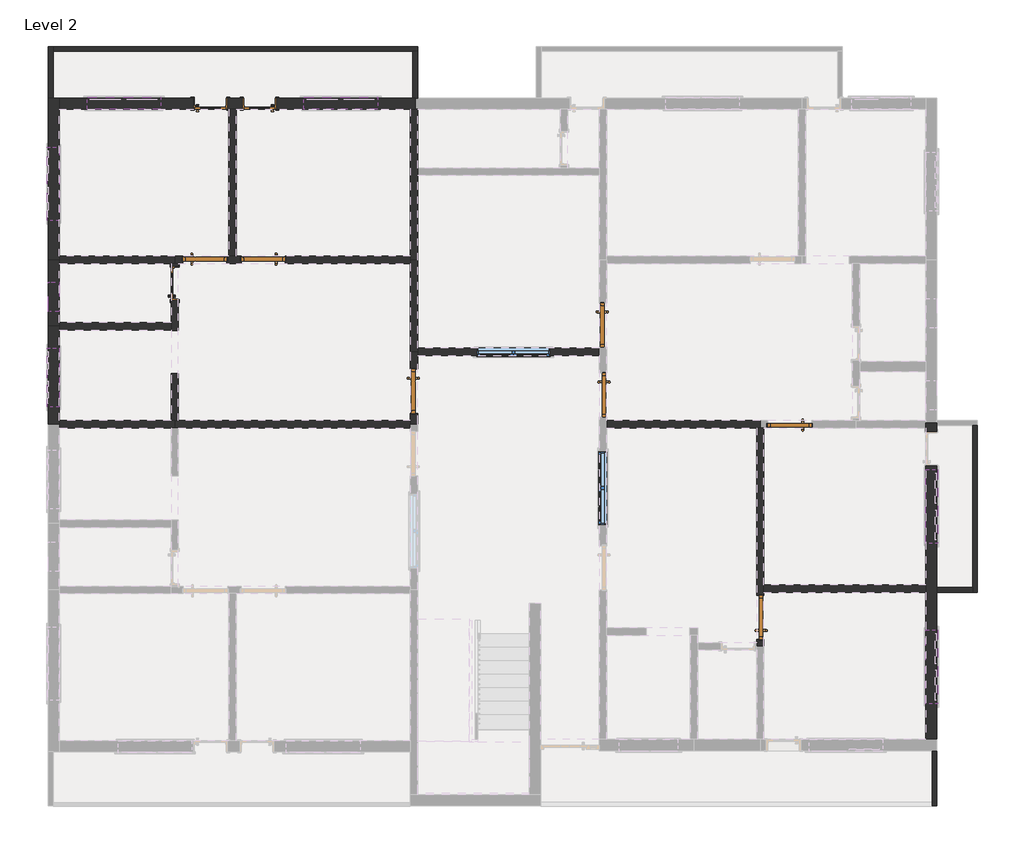
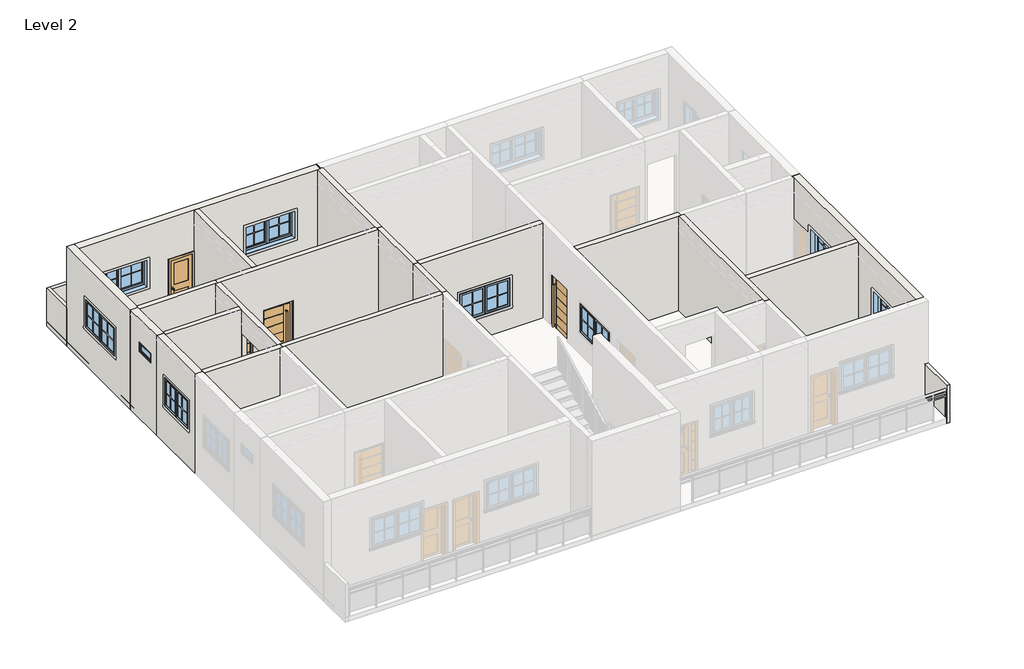
# One storey, part 2 of 5: 25 walls, 10 doors, 9 windows.
"""IFC4 building model written with IfcOpenShell, lengths in millimetres."""

from ifc_helpers import new_model, si_unit, frame, origin, place, context, project, spatial, polyline, outline, extrude, faceted_brep, transform, mapped, element, save
from components import door_3_ad1505b7, door_3_44036f4b, door_57d9c04c, door_5f4ff63b, door_e2914254, fixed_2_d9cafb20, m_window_awning_double_horizontal_4_0c6a2509, m_window_awning_double_horizontal_5_7c720334, m_window_awning_double_horizontal_5_337400f2

model = new_model("IFC4")

# Units and contexts
model_context = context("Model", 3, world=origin())
ifc_project = project(units=[si_unit("LENGTHUNIT", "METRE", prefix="MILLI")], contexts=[model_context])

# Site, building, storey
site = spatial("IfcSite", under=ifc_project)
building = spatial("IfcBuilding", under=site)
storey = spatial("IfcBuildingStorey", under=building, Name="Level 2", Elevation=3200.4)

# Doors
placement = place(None, origin())
door_3_shape = door_3_ad1505b7(model_context)
element("IfcDoor", 1, ObjectType="3'", at=placement, inside=storey, context=model_context, shape_type="MappedRepresentation", body=[
    mapped(door_3_shape, transform((-21766.1847893, 19978.1922903, 3200.4), x_axis=(1.0, 0.0, 0.0), y_axis=(0.0, 1.0, 0.0), z_axis=(0.0, 0.0, 1.0))),
])
element("IfcDoor", 2, ObjectType="3'", at=placement, inside=storey, context=model_context, shape_type="MappedRepresentation", body=[
    mapped(door_3_shape, transform((-13523.8847893, 17184.1922903, 3200.4), x_axis=(0.0, -1.0, 0.0), y_axis=(1.0, 0.0, 0.0), z_axis=(0.0, 0.0, 1.0))),
])
element("IfcDoor", 3, ObjectType="3'", at=placement, inside=storey, context=model_context, shape_type="MappedRepresentation", body=[
    mapped(door_3_shape, transform((-9663.0847893, 16574.5922903, 3200.4), x_axis=(-1.0, 0.0, 0.0), y_axis=(0.0, -1.0, 0.0), z_axis=(0.0, 0.0, 1.0))),
])
door_3_2_shape = door_3_44036f4b(model_context)
element("IfcDoor", 4, ObjectType="3'", at=placement, inside=storey, context=model_context, shape_type="MappedRepresentation", body=[
    mapped(door_3_2_shape, transform((-20559.6847893, 19978.1922903, 3200.4), x_axis=(-1.0, 0.0, 0.0), y_axis=(0.0, -1.0, 0.0), z_axis=(0.0, 0.0, 1.0))),
])
element("IfcDoor", 5, ObjectType="3'", at=placement, inside=storey, context=model_context, shape_type="MappedRepresentation", body=[
    mapped(door_3_2_shape, transform((-17435.4847893, 17260.3922903, 3200.4), x_axis=(0.0, -1.0, 0.0), y_axis=(1.0, 0.0, 0.0), z_axis=(0.0, 0.0, 1.0))),
])
element("IfcDoor", 6, ObjectType="3'", at=placement, inside=storey, context=model_context, shape_type="MappedRepresentation", body=[
    mapped(door_3_2_shape, transform((-13523.8847893, 18631.9922903, 3200.4), x_axis=(0.0, -1.0, 0.0), y_axis=(1.0, 0.0, 0.0), z_axis=(0.0, 0.0, 1.0))),
])
element("IfcDoor", 7, ObjectType="3'", at=placement, inside=storey, context=model_context, shape_type="MappedRepresentation", body=[
    mapped(door_3_2_shape, transform((-10272.6847893, 12574.0922903, 3200.4), x_axis=(0.0, 1.0, 0.0), y_axis=(-1.0, 0.0, 0.0), z_axis=(0.0, 0.0, 1.0))),
])
door_shape = door_57d9c04c(model_context)
element("IfcDoor", 8, ObjectType="M_Door-Interior-Single-2_Panel-Wood : 2'2\"", at=placement, inside=storey, context=model_context, shape_type="MappedRepresentation", body=[
    mapped(door_shape, transform((-22391.6597893, 19495.5922903, 3200.4), x_axis=(0.0, 1.0, 0.0), y_axis=(-1.0, 0.0, 0.0), z_axis=(0.0, 0.0, 1.0))),
])
door_2_shape = door_5f4ff63b(model_context)
element("IfcDoor", 9, ObjectType="M_Door-Interior-Single-2_Panel-Wood : 2'2\"", at=placement, inside=storey, context=model_context, shape_type="MappedRepresentation", body=[
    mapped(door_2_shape, transform((-20635.8847893, 23213.5172903, 3200.4), x_axis=(-1.0, 0.0, 0.0), y_axis=(0.0, -1.0, 0.0), z_axis=(0.0, 0.0, 1.0))),
])
door_4_shape = door_e2914254(model_context)
element("IfcDoor", 10, ObjectType="M_Door-Interior-Single-2_Panel-Wood : 2'2\"", at=placement, inside=storey, context=model_context, shape_type="MappedRepresentation", body=[
    mapped(door_4_shape, transform((-21651.8847893, 23213.5172903, 3200.4), x_axis=(1.0, 0.0, 0.0), y_axis=(0.0, 1.0, 0.0), z_axis=(0.0, 0.0, 1.0))),
])

# Walls
element("IfcWall", 11, ObjectType="Generic - 4\"", at=placement, inside=storey, context=model_context, shape_type="Brep", body=[
    faceted_brep([(-24903.0847893, 23330.9922903, 3200.4), (-24903.0847893, 24296.1922903, 3200.4), (-24903.0847893, 24397.7922903, 3200.4), (-24903.0847893, 24397.7922903, 4419.6), (-24903.0847893, 24296.1922903, 4419.6), (-24903.0847893, 23330.9922903, 4419.6), (-25004.6847893, 23330.9922903, 3200.4), (-25004.6847893, 23330.9922903, 4419.6), (-25004.6847893, 24397.7922903, 4419.6), (-25004.6847893, 24397.7922903, 3200.4)], [[[0, 1, 2, 3, 4, 5]], [[6, 7, 8, 9]], [[2, 1, 0, 6, 9]], [[5, 4, 3, 8, 7]], [[0, 5, 7, 6]], [[3, 2, 9, 8]]]),
])
element("IfcWall", 12, ObjectType="Generic - 4\"", at=placement, inside=storey, context=model_context, shape_type="Brep", body=[
    faceted_brep([(-24903.0847893, 24296.1922903, 3200.4), (-17460.8847893, 24296.1922903, 3200.4), (-17359.2847893, 24296.1922903, 3200.4), (-17359.2847893, 24296.1922903, 4419.6), (-17460.8847893, 24296.1922903, 4419.6), (-24903.0847893, 24296.1922903, 4419.6), (-24903.0847893, 24397.7922903, 3200.4), (-24903.0847893, 24397.7922903, 4419.6), (-17359.2847893, 24397.7922903, 4419.6), (-17359.2847893, 24397.7922903, 3200.4)], [[[0, 1, 2, 3, 4, 5]], [[6, 7, 8, 9]], [[2, 1, 0, 6, 9]], [[5, 4, 3, 8, 7]], [[0, 5, 7, 6]], [[3, 2, 9, 8]]]),
])
element("IfcWall", 13, ObjectType="Generic - 4\"", at=placement, inside=storey, context=model_context, shape_type="Brep", body=[
    faceted_brep([(-17460.8847893, 24296.1922903, 3200.4), (-17460.8847893, 23330.9922903, 3200.4), (-17460.8847893, 23330.9922903, 4419.6), (-17460.8847893, 24296.1922903, 4419.6), (-17359.2847893, 24296.1922903, 3200.4), (-17359.2847893, 24296.1922903, 4419.6), (-17359.2847893, 23330.9922903, 4419.6), (-17359.2847893, 23330.9922903, 3200.4), (-17410.0847893, 23330.9922903, 3200.4), (-17435.4847893, 23330.9922903, 3200.4)], [[[0, 1, 2, 3]], [[4, 5, 6, 7]], [[1, 0, 4, 7, 8, 9]], [[3, 2, 6, 5]], [[0, 3, 5, 4]], [[2, 1, 9, 8, 7, 6]]]),
])
element("IfcWall", 14, ObjectType="Generic - 4\"", at=placement, inside=storey, context=model_context, shape_type="Brep", body=[
    faceted_brep([(-5878.4847893, 16549.1922903, 3200.4), (-5878.4847893, 13196.3922903, 3200.4), (-5878.4847893, 13094.7922903, 3200.4), (-5878.4847893, 13094.7922903, 4419.6), (-5878.4847893, 13196.3922903, 4419.6), (-5878.4847893, 16549.1922903, 4419.6), (-5776.8847893, 16549.1922903, 3200.4), (-5776.8847893, 16549.1922903, 4419.6), (-5776.8847893, 13094.7922903, 4419.6), (-5776.8847893, 13094.7922903, 3200.4)], [[[0, 1, 2, 3, 4, 5]], [[6, 7, 8, 9]], [[2, 1, 0, 6, 9]], [[5, 4, 3, 8, 7]], [[0, 5, 7, 6]], [[3, 2, 9, 8]]]),
])
element("IfcWall", 15, ObjectType="Generic - 4\"", at=placement, inside=storey, context=model_context, shape_type="SweptSolid", body=[
    extrude(outline(polyline([(-6615.0847893, 13196.3922903), (-5878.4847893, 13196.3922903), (-5878.4847893, 13094.7922903), (-6615.0847893, 13094.7922903), (-6615.0847893, 13196.3922903)])), frame((0.0, 0.0, 3200.4), z_axis=(0.0, 0.0, 1.0), x_axis=(1.0, 0.0, 0.0)), (0.0, 0.0, 1.0), 1219.2),
])
element("IfcWall", 16, ObjectType="Generic - 4\"", at=placement, inside=storey, context=model_context, shape_type="SweptSolid", body=[
    extrude(outline(polyline([(-6716.6847893, 8675.1922903), (-6716.6847893, 9818.1922903), (-6615.0847893, 9818.1922903), (-6615.0847893, 8675.1922903), (-6716.6847893, 8675.1922903)])), frame((0.0, 0.0, 3200.4), z_axis=(0.0, 0.0, 1.0), x_axis=(1.0, 0.0, 0.0)), (0.0, 0.0, 1.0), 1219.2),
])
element("IfcWall", 17, ObjectType="Generic - 6\"", at=placement, inside=storey, context=model_context, shape_type="Brep", body=[
    faceted_brep([(-17511.6847893, 23102.3922903, 6400.8), (-17511.6847893, 23102.3922903, 3200.4), (-17511.6847893, 20054.3922903, 3200.4), (-17511.6847893, 19978.1922903, 3200.4), (-17511.6847893, 19978.1922903, 6400.8), (-17511.6847893, 20054.3922903, 6400.8), (-17359.2847893, 23102.3922903, 3200.4), (-17359.2847893, 23102.3922903, 6400.8), (-17359.2847893, 21883.1922903, 6400.8), (-17359.2847893, 21730.7922903, 6400.8), (-17359.2847893, 19978.1922903, 6400.8), (-17359.2847893, 19978.1922903, 3200.4), (-17359.2847893, 21730.7922903, 3200.4), (-17359.2847893, 21883.1922903, 3200.4), (-17435.4847893, 23102.3922903, 3200.4), (-17410.0847893, 23102.3922903, 3200.4), (-17410.0847893, 23102.3922903, 6400.8), (-17435.4847893, 23102.3922903, 6400.8)], [[[0, 1, 2, 3, 4, 5]], [[6, 7, 8, 9, 10, 11, 12, 13]], [[3, 2, 1, 14, 15, 6, 13, 12, 11]], [[4, 3, 11, 10]], [[0, 5, 4, 10, 9, 8, 7, 16, 17]], [[0, 17, 16, 7, 6, 15, 14, 1]]]),
])
element("IfcWall", 18, ObjectType="Generic - 6\"", at=placement, inside=storey, context=model_context, shape_type="Brep", body=[
    faceted_brep([(-24776.0847893, 19901.9922903, 3200.4), (-22464.6847893, 19901.9922903, 3200.4), (-22388.4847893, 19901.9922903, 3200.4), (-22388.4847893, 19901.9922903, 6400.8), (-22464.6847893, 19901.9922903, 6400.8), (-24776.0847893, 19901.9922903, 6400.8), (-24776.0847893, 20054.3922903, 3200.4), (-24776.0847893, 20054.3922903, 6400.8), (-22388.4847893, 20054.3922903, 6400.8), (-22388.4847893, 20054.3922903, 3200.4), (-24776.0847893, 19978.1922903, 3200.4), (-24776.0847893, 19978.1922903, 6400.8)], [[[0, 1, 2, 3, 4, 5]], [[6, 7, 8, 9]], [[2, 1, 0, 10, 6, 9]], [[3, 2, 9, 8]], [[5, 4, 3, 8, 7, 11]], [[0, 5, 11, 7, 6, 10]]]),
])
element("IfcWall", 19, ObjectType="Generic - 6\"", at=placement, inside=storey, context=model_context, shape_type="SweptSolid", body=[
    extrude(outline(polyline([(-21270.8847893, 20054.3922903), (-21270.8847893, 23102.3922903), (-21118.4847893, 23102.3922903), (-21118.4847893, 20054.3922903), (-21270.8847893, 20054.3922903)])), frame((0.0, 0.0, 3200.4), z_axis=(0.0, 0.0, 1.0), x_axis=(1.0, 0.0, 0.0)), (0.0, 0.0, 1.0), 3200.4),
])
element("IfcWall", 20, ObjectType="Generic - 6\"", at=placement, inside=storey, context=model_context, shape_type="Brep", body=[
    faceted_brep([(-24776.0847893, 16498.3922903, 3200.4), (-22464.6847893, 16498.3922903, 3200.4), (-22388.4847893, 16498.3922903, 3200.4), (-22388.4847893, 16498.3922903, 6400.8), (-22464.6847893, 16498.3922903, 6400.8), (-24776.0847893, 16498.3922903, 6400.8), (-24776.0847893, 16650.7922903, 3200.4), (-24776.0847893, 16650.7922903, 6400.8), (-22464.6847893, 16650.7922903, 6400.8), (-22388.4847893, 16650.7922903, 6400.8), (-22388.4847893, 16650.7922903, 3200.4), (-22464.6847893, 16650.7922903, 3200.4), (-24776.0847893, 16574.5922903, 3200.4), (-24776.0847893, 16574.5922903, 6400.8)], [[[0, 1, 2, 3, 4, 5]], [[6, 7, 8, 9, 10, 11]], [[2, 1, 0, 12, 6, 11, 10]], [[3, 2, 10, 9]], [[5, 4, 3, 9, 8, 7, 13]], [[0, 5, 13, 7, 6, 12]]]),
])
element("IfcWall", 21, ObjectType="Generic - 6\"", at=placement, inside=storey, context=model_context, shape_type="Brep", body=[
    faceted_brep([(-24776.0847893, 18530.3922903, 3200.4), (-22464.6847893, 18530.3922903, 3200.4), (-22464.6847893, 18530.3922903, 6400.8), (-24776.0847893, 18530.3922903, 6400.8), (-24776.0847893, 18682.7922903, 3200.4), (-24776.0847893, 18682.7922903, 6400.8), (-22464.6847893, 18682.7922903, 6400.8), (-22464.6847893, 18682.7922903, 3200.4), (-24776.0847893, 18606.5922903, 3200.4), (-24776.0847893, 18606.5922903, 6400.8)], [[[0, 1, 2, 3]], [[4, 5, 6, 7]], [[1, 0, 8, 4, 7]], [[3, 2, 6, 5, 9]], [[0, 3, 9, 5, 4, 8]], [[2, 1, 7, 6]]]),
])
element("IfcWall", 22, ObjectType="Generic - 6\"", at=placement, inside=storey, context=model_context, shape_type="Brep", body=[
    faceted_brep([(-22312.2847893, 19901.9922903, 6400.8), (-22312.2847893, 16650.7922903, 6400.8), (-22312.2847893, 16650.7922903, 3200.4), (-22312.2847893, 17622.2018411, 3200.4), (-22312.2847893, 17622.2018411, 5638.8), (-22312.2847893, 18518.7795946, 5638.8), (-22312.2847893, 18518.7795946, 3200.4), (-22312.2847893, 19140.3922903, 3200.4), (-22312.2847893, 19140.3922903, 5054.2), (-22312.2847893, 19850.7922903, 5054.2), (-22312.2847893, 19850.7922903, 3200.4), (-22312.2847893, 19901.9922903, 3200.4), (-22464.6847893, 16650.7922903, 6400.8), (-22464.6847893, 18530.3922903, 6400.8), (-22464.6847893, 18682.7922903, 6400.8), (-22464.6847893, 19901.9922903, 6400.8), (-22464.6847893, 19901.9922903, 3200.4), (-22464.6847893, 19850.7922903, 3200.4), (-22464.6847893, 19850.7922903, 5054.2), (-22464.6847893, 19140.3922903, 5054.2), (-22464.6847893, 19140.3922903, 3200.4), (-22464.6847893, 18682.7922903, 3200.4), (-22464.6847893, 18530.3922903, 3200.4), (-22464.6847893, 18518.7795946, 3200.4), (-22464.6847893, 18518.7795946, 5638.8), (-22464.6847893, 17622.2018411, 5638.8), (-22464.6847893, 17622.2018411, 3200.4), (-22464.6847893, 16650.7922903, 3200.4), (-22388.4847893, 16650.7922903, 3200.4), (-22388.4847893, 19901.9922903, 3200.4), (-22388.4847893, 19901.9922903, 6400.8), (-22388.4847893, 16650.7922903, 6400.8)], [[[0, 1, 2, 3, 4, 5, 6, 7, 8, 9, 10, 11]], [[12, 13, 14, 15, 16, 17, 18, 19, 20, 21, 22, 23, 24, 25, 26, 27]], [[2, 28, 27, 26, 3]], [[6, 23, 22, 21, 20, 7]], [[16, 29, 11, 10, 17]], [[1, 0, 30, 15, 14, 13, 12, 31]], [[0, 11, 29, 16, 15, 30]], [[2, 1, 31, 12, 27, 28]], [[9, 18, 17, 10]], [[18, 9, 8, 19]], [[19, 8, 7, 20]], [[4, 25, 24, 5]], [[25, 4, 3, 26]], [[5, 24, 23, 6]]]),
])
element("IfcWall", 23, ObjectType="Generic - 6\"", at=placement, inside=storey, context=model_context, shape_type="Brep", body=[
    faceted_brep([(-17359.2847893, 17996.9922903, 3200.4), (-13600.0847893, 17996.9922903, 3200.4), (-13600.0847893, 17996.9922903, 6400.8), (-17359.2847893, 17996.9922903, 6400.8), (-16140.0847893, 17996.9922903, 5014.8), (-14616.0847893, 17996.9922903, 5014.8), (-14616.0847893, 17996.9922903, 4100.4), (-16140.0847893, 17996.9922903, 4100.4), (-17359.2847893, 18149.3922903, 3200.4), (-17359.2847893, 18149.3922903, 6400.8), (-13600.0847893, 18149.3922903, 6400.8), (-13600.0847893, 18149.3922903, 3200.4), (-16140.0847893, 18149.3922903, 5014.8), (-16140.0847893, 18149.3922903, 4100.4), (-14616.0847893, 18149.3922903, 4100.4), (-14616.0847893, 18149.3922903, 5014.8), (-17359.2847893, 18073.1922903, 3200.4), (-17359.2847893, 18073.1922903, 6400.8)], [[[0, 1, 2, 3], [4, 5, 6, 7]], [[8, 9, 10, 11], [12, 13, 14, 15]], [[1, 0, 16, 8, 11]], [[3, 2, 10, 9, 17]], [[0, 3, 17, 9, 8, 16]], [[2, 1, 11, 10]], [[13, 12, 4, 7]], [[14, 13, 7, 6]], [[15, 14, 6, 5]], [[12, 15, 5, 4]]]),
])
element("IfcWall", 24, ObjectType="Generic - 6\"", at=placement, inside=storey, context=model_context, shape_type="Brep", body=[
    faceted_brep([(-13447.6847893, 16498.3922903, 3200.4), (-10348.8847893, 16498.3922903, 3200.4), (-10272.6847893, 16498.3922903, 3200.4), (-10272.6847893, 16498.3922903, 6400.8), (-10348.8847893, 16498.3922903, 6400.8), (-13447.6847893, 16498.3922903, 6400.8), (-13447.6847893, 16650.7922903, 3200.4), (-13447.6847893, 16650.7922903, 6400.8), (-10272.6847893, 16650.7922903, 6400.8), (-10272.6847893, 16650.7922903, 3200.4)], [[[0, 1, 2, 3, 4, 5]], [[6, 7, 8, 9]], [[2, 1, 0, 6, 9]], [[3, 2, 9, 8]], [[5, 4, 3, 8, 7]], [[0, 5, 7, 6]]]),
])
element("IfcWall", 25, ObjectType="Generic - 6\"", at=placement, inside=storey, context=model_context, shape_type="Brep", body=[
    faceted_brep([(-10348.8847893, 11977.1922903, 3200.4), (-10348.8847893, 11977.1922903, 6400.8), (-10348.8847893, 12053.3922903, 6400.8), (-10348.8847893, 16498.3922903, 6400.8), (-10348.8847893, 16498.3922903, 3200.4), (-10348.8847893, 13031.2922903, 3200.4), (-10348.8847893, 13031.2922903, 5029.2), (-10348.8847893, 12116.8922903, 5029.2), (-10348.8847893, 12116.8922903, 3200.4), (-10348.8847893, 12053.3922903, 3200.4), (-10196.4847893, 11977.1922903, 6400.8), (-10196.4847893, 11977.1922903, 3200.4), (-10196.4847893, 12116.8922903, 3200.4), (-10196.4847893, 12116.8922903, 5029.2), (-10196.4847893, 13031.2922903, 5029.2), (-10196.4847893, 13031.2922903, 3200.4), (-10196.4847893, 13094.7922903, 3200.4), (-10196.4847893, 13247.1922903, 3200.4), (-10196.4847893, 16498.3922903, 3200.4), (-10196.4847893, 16498.3922903, 6400.8), (-10196.4847893, 13247.1922903, 6400.8), (-10196.4847893, 13094.7922903, 6400.8), (-10272.6847893, 16498.3922903, 3200.4), (-10216.4847893, 13031.2922903, 3200.4), (-10216.4847893, 13046.2922903, 3200.4), (-10293.4847893, 13046.2922903, 3200.4), (-10293.4847893, 13031.2922903, 3200.4), (-10293.4847893, 12116.8922903, 3200.4), (-10293.4847893, 12101.8922903, 3200.4), (-10216.4847893, 12101.8922903, 3200.4), (-10216.4847893, 12116.8922903, 3200.4), (-10272.6847893, 16498.3922903, 6400.8), (-10216.4847893, 12116.8922903, 5029.2), (-10216.4847893, 13031.2922903, 5029.2), (-10293.4847893, 13031.2922903, 5029.2), (-10293.4847893, 12116.8922903, 5029.2), (-10216.4847893, 12101.8922903, 5044.2), (-10293.4847893, 12101.8922903, 5044.2), (-10293.4847893, 13046.2922903, 5044.2), (-10216.4847893, 13046.2922903, 5044.2)], [[[0, 1, 2, 3, 4, 5, 6, 7, 8, 9]], [[10, 11, 12, 13, 14, 15, 16, 17, 18, 19, 20, 21]], [[4, 22, 18, 17, 16, 15, 23, 24, 25, 26, 5]], [[11, 0, 9, 8, 27, 28, 29, 30, 12]], [[1, 0, 11, 10]], [[3, 2, 1, 10, 21, 20, 19, 31]], [[4, 3, 31, 19, 18, 22]], [[13, 32, 33, 14]], [[6, 34, 35, 7]], [[14, 33, 23, 15]], [[34, 6, 5, 26]], [[32, 13, 12, 30]], [[7, 35, 27, 8]], [[36, 37, 38, 39]], [[39, 38, 25, 24]], [[35, 34, 26, 25, 38, 37, 28, 27]], [[37, 36, 29, 28]], [[33, 32, 30, 29, 36, 39, 24, 23]]]),
])
element("IfcWall", 26, ObjectType="Generic - 6\"", at=placement, inside=storey, context=model_context, shape_type="SweptSolid", body=[
    extrude(outline(polyline([(-6843.6847893, 13094.7922903), (-10196.4847893, 13094.7922903), (-10196.4847893, 13247.1922903), (-6843.6847893, 13247.1922903), (-6843.6847893, 13094.7922903)])), frame((0.0, 0.0, 3200.4), z_axis=(0.0, 0.0, 1.0), x_axis=(1.0, 0.0, 0.0)), (0.0, 0.0, 1.0), 3200.4),
])
element("IfcWall", 27, ObjectType="Generic - 6\"", at=placement, inside=storey, context=model_context, shape_type="Brep", body=[
    faceted_brep([(-22388.4847893, 16498.3922903, 3200.4), (-22312.2847893, 16498.3922903, 3200.4), (-17511.6847893, 16498.3922903, 3200.4), (-17511.6847893, 16498.3922903, 6400.8), (-22312.2847893, 16498.3922903, 6400.8), (-22388.4847893, 16498.3922903, 6400.8), (-22388.4847893, 16650.7922903, 3200.4), (-22388.4847893, 16650.7922903, 6400.8), (-22312.2847893, 16650.7922903, 6400.8), (-17511.6847893, 16650.7922903, 6400.8), (-17511.6847893, 16650.7922903, 3200.4), (-22312.2847893, 16650.7922903, 3200.4), (-17511.6847893, 16574.5922903, 3200.4), (-17511.6847893, 16574.5922903, 6400.8)], [[[0, 1, 2, 3, 4, 5]], [[6, 7, 8, 9, 10, 11]], [[2, 1, 0, 6, 11, 10, 12]], [[5, 4, 3, 13, 9, 8, 7]], [[0, 5, 7, 6]], [[3, 2, 12, 10, 9, 13]]]),
])
element("IfcWall", 28, ObjectType="Generic - 6\"", at=placement, inside=storey, context=model_context, shape_type="Brep", body=[
    faceted_brep([(-17511.6847893, 19978.1922903, 3200.4), (-17511.6847893, 19901.9922903, 3200.4), (-17511.6847893, 18073.1922903, 3200.4), (-17511.6847893, 18073.1922903, 6400.8), (-17511.6847893, 19901.9922903, 6400.8), (-17511.6847893, 19978.1922903, 6400.8), (-17359.2847893, 19978.1922903, 3200.4), (-17359.2847893, 19978.1922903, 6400.8), (-17359.2847893, 18149.3922903, 6400.8), (-17359.2847893, 18073.1922903, 6400.8), (-17359.2847893, 18073.1922903, 3200.4), (-17359.2847893, 18149.3922903, 3200.4)], [[[0, 1, 2, 3, 4, 5]], [[6, 7, 8, 9, 10, 11]], [[2, 1, 0, 6, 11, 10]], [[3, 2, 10, 9]], [[5, 4, 3, 9, 8, 7]], [[0, 5, 7, 6]]]),
])
element("IfcWall", 29, ObjectType="Generic - 6\"", at=placement, inside=storey, context=model_context, shape_type="Brep", body=[
    faceted_brep([(-17511.6847893, 19901.9922903, 6400.8), (-22312.2847893, 19901.9922903, 6400.8), (-22388.4847893, 19901.9922903, 6400.8), (-22388.4847893, 19901.9922903, 3200.4), (-22312.2847893, 19901.9922903, 3200.4), (-22223.3847893, 19901.9922903, 3200.4), (-22223.3847893, 19901.9922903, 5029.2), (-21308.9847893, 19901.9922903, 5029.2), (-21308.9847893, 19901.9922903, 3200.4), (-21016.8847893, 19901.9922903, 3200.4), (-21016.8847893, 19901.9922903, 5029.2), (-20102.4847893, 19901.9922903, 5029.2), (-20102.4847893, 19901.9922903, 3200.4), (-17511.6847893, 19901.9922903, 3200.4), (-22388.4847893, 20054.3922903, 6400.8), (-21270.8847893, 20054.3922903, 6400.8), (-21118.4847893, 20054.3922903, 6400.8), (-17511.6847893, 20054.3922903, 6400.8), (-17511.6847893, 20054.3922903, 3200.4), (-20102.4847893, 20054.3922903, 3200.4), (-20102.4847893, 20054.3922903, 5029.2), (-21016.8847893, 20054.3922903, 5029.2), (-21016.8847893, 20054.3922903, 3200.4), (-21118.4847893, 20054.3922903, 3200.4), (-21270.8847893, 20054.3922903, 3200.4), (-21308.9847893, 20054.3922903, 3200.4), (-21308.9847893, 20054.3922903, 5029.2), (-22223.3847893, 20054.3922903, 5029.2), (-22223.3847893, 20054.3922903, 3200.4), (-22388.4847893, 20054.3922903, 3200.4), (-17511.6847893, 19978.1922903, 3200.4), (-20102.4847893, 19957.3922903, 3200.4), (-20087.4847893, 19957.3922903, 3200.4), (-20087.4847893, 20034.3922903, 3200.4), (-20102.4847893, 20034.3922903, 3200.4), (-21308.9847893, 19957.3922903, 3200.4), (-21293.9847893, 19957.3922903, 3200.4), (-21293.9847893, 20034.3922903, 3200.4), (-21308.9847893, 20034.3922903, 3200.4), (-21016.8847893, 20034.3922903, 3200.4), (-21031.8847893, 20034.3922903, 3200.4), (-21031.8847893, 19957.3922903, 3200.4), (-21016.8847893, 19957.3922903, 3200.4), (-22223.3847893, 20034.3922903, 3200.4), (-22238.3847893, 20034.3922903, 3200.4), (-22238.3847893, 19957.3922903, 3200.4), (-22223.3847893, 19957.3922903, 3200.4), (-17511.6847893, 19978.1922903, 6400.8), (-22223.3847893, 19957.3922903, 5029.2), (-21308.9847893, 19957.3922903, 5029.2), (-22223.3847893, 20034.3922903, 5029.2), (-21308.9847893, 20034.3922903, 5029.2), (-22238.3847893, 20034.3922903, 5044.2), (-21293.9847893, 20034.3922903, 5044.2), (-21293.9847893, 19957.3922903, 5044.2), (-22238.3847893, 19957.3922903, 5044.2), (-20102.4847893, 20034.3922903, 5029.2), (-21016.8847893, 20034.3922903, 5029.2), (-21016.8847893, 19957.3922903, 5029.2), (-20102.4847893, 19957.3922903, 5029.2), (-20087.4847893, 20034.3922903, 5044.2), (-20087.4847893, 19957.3922903, 5044.2), (-21031.8847893, 19957.3922903, 5044.2), (-21031.8847893, 20034.3922903, 5044.2)], [[[0, 1, 2, 3, 4, 5, 6, 7, 8, 9, 10, 11, 12, 13]], [[14, 15, 16, 17, 18, 19, 20, 21, 22, 23, 24, 25, 26, 27, 28, 29]], [[18, 30, 13, 12, 31, 32, 33, 34, 19]], [[8, 35, 36, 37, 38, 25, 24, 23, 22, 39, 40, 41, 42, 9]], [[3, 29, 28, 43, 44, 45, 46, 5, 4]], [[2, 1, 0, 47, 17, 16, 15, 14]], [[3, 2, 14, 29]], [[0, 13, 30, 18, 17, 47]], [[6, 48, 49, 7]], [[50, 27, 26, 51]], [[7, 49, 35, 8]], [[51, 26, 25, 38]], [[48, 6, 5, 46]], [[27, 50, 43, 28]], [[52, 53, 54, 55]], [[54, 53, 37, 36]], [[55, 54, 36, 35, 49, 48, 46, 45]], [[52, 55, 45, 44]], [[53, 52, 44, 43, 50, 51, 38, 37]], [[20, 56, 57, 21]], [[10, 58, 59, 11]], [[58, 10, 9, 42]], [[21, 57, 39, 22]], [[11, 59, 31, 12]], [[56, 20, 19, 34]], [[60, 61, 62, 63]], [[63, 62, 41, 40]], [[59, 58, 42, 41, 62, 61, 32, 31]], [[61, 60, 33, 32]], [[57, 56, 34, 33, 60, 63, 40, 39]]]),
])
element("IfcWall", 30, ObjectType="Generic - 6\"", at=placement, inside=storey, context=model_context, shape_type="Brep", body=[
    faceted_brep([(-17511.6847893, 16574.5922903, 3200.4), (-17511.6847893, 16574.5922903, 6400.8), (-17511.6847893, 16650.7922903, 6400.8), (-17511.6847893, 18073.1922903, 6400.8), (-17511.6847893, 18073.1922903, 3200.4), (-17511.6847893, 17717.5922903, 3200.4), (-17511.6847893, 17717.5922903, 5029.2), (-17511.6847893, 16803.1922903, 5029.2), (-17511.6847893, 16803.1922903, 3200.4), (-17511.6847893, 16650.7922903, 3200.4), (-17359.2847893, 16574.5922903, 6400.8), (-17359.2847893, 16574.5922903, 3200.4), (-17359.2847893, 16803.1922903, 3200.4), (-17359.2847893, 16803.1922903, 5029.2), (-17359.2847893, 17717.5922903, 5029.2), (-17359.2847893, 17717.5922903, 3200.4), (-17359.2847893, 17996.9922903, 3200.4), (-17359.2847893, 18073.1922903, 3200.4), (-17359.2847893, 18073.1922903, 6400.8), (-17359.2847893, 17996.9922903, 6400.8), (-17414.6847893, 17717.5922903, 3200.4), (-17414.6847893, 17732.5922903, 3200.4), (-17491.6847893, 17732.5922903, 3200.4), (-17491.6847893, 17717.5922903, 3200.4), (-17491.6847893, 16803.1922903, 3200.4), (-17491.6847893, 16788.1922903, 3200.4), (-17414.6847893, 16788.1922903, 3200.4), (-17414.6847893, 16803.1922903, 3200.4), (-17491.6847893, 17717.5922903, 5029.2), (-17491.6847893, 16803.1922903, 5029.2), (-17414.6847893, 16803.1922903, 5029.2), (-17414.6847893, 17717.5922903, 5029.2), (-17491.6847893, 17732.5922903, 5044.2), (-17414.6847893, 17732.5922903, 5044.2), (-17414.6847893, 16788.1922903, 5044.2), (-17491.6847893, 16788.1922903, 5044.2)], [[[0, 1, 2, 3, 4, 5, 6, 7, 8, 9]], [[10, 11, 12, 13, 14, 15, 16, 17, 18, 19]], [[4, 17, 16, 15, 20, 21, 22, 23, 5]], [[11, 0, 9, 8, 24, 25, 26, 27, 12]], [[1, 0, 11, 10]], [[3, 2, 1, 10, 19, 18]], [[4, 3, 18, 17]], [[6, 28, 29, 7]], [[13, 30, 31, 14]], [[30, 13, 12, 27]], [[7, 29, 24, 8]], [[14, 31, 20, 15]], [[28, 6, 5, 23]], [[32, 33, 34, 35]], [[35, 34, 26, 25]], [[31, 30, 27, 26, 34, 33, 21, 20]], [[33, 32, 22, 21]], [[29, 28, 23, 22, 32, 35, 25, 24]]]),
])
element("IfcWall", 31, ObjectType="Generic - 9\"", at=placement, inside=storey, context=model_context, shape_type="Brep", body=[
    faceted_brep([(-25004.6847893, 23330.9922903, 6400.8), (-25004.6847893, 23330.9922903, 4419.6), (-25004.6847893, 23330.9922903, 3200.4), (-25004.6847893, 19978.1922903, 3200.4), (-25004.6847893, 19978.1922903, 6400.8), (-25004.6847893, 22314.9922903, 5333.9570313), (-25004.6847893, 20790.9922903, 5333.9570313), (-25004.6847893, 20790.9922903, 4419.5570313), (-25004.6847893, 22314.9922903, 4419.5570313), (-24776.0847893, 23330.9922903, 3200.4), (-24776.0847893, 23330.9922903, 6400.8), (-24776.0847893, 23102.3922903, 6400.8), (-24776.0847893, 20054.3922903, 6400.8), (-24776.0847893, 19978.1922903, 6400.8), (-24776.0847893, 19978.1922903, 3200.4), (-24776.0847893, 20054.3922903, 3200.4), (-24776.0847893, 23102.3922903, 3200.4), (-24776.0847893, 22314.9922903, 5333.9570313), (-24776.0847893, 22314.9922903, 4419.5570313), (-24776.0847893, 20790.9922903, 4419.5570313), (-24776.0847893, 20790.9922903, 5333.9570313), (-24903.0847893, 23330.9922903, 3200.4)], [[[0, 1, 2, 3, 4], [5, 6, 7, 8]], [[9, 10, 11, 12, 13, 14, 15, 16], [17, 18, 19, 20]], [[3, 2, 21, 9, 16, 15, 14]], [[4, 3, 14, 13]], [[0, 4, 13, 12, 11, 10]], [[18, 17, 5, 8]], [[19, 18, 8, 7]], [[20, 19, 7, 6]], [[17, 20, 6, 5]], [[0, 10, 9, 21, 2, 1]]]),
])
element("IfcWall", 32, ObjectType="Generic - 9\"", at=placement, inside=storey, context=model_context, shape_type="Brep", body=[
    faceted_brep([(-6615.0847893, 16599.9922903, 6400.8), (-6615.0847893, 10046.7922903, 6400.8), (-6615.0847893, 10046.7922903, 3200.4), (-6615.0847893, 13094.7922903, 3200.4), (-6615.0847893, 13196.3922903, 3200.4), (-6615.0847893, 15711.3922903, 3200.4), (-6615.0847893, 15711.3922903, 5054.2), (-6615.0847893, 16421.7922903, 5054.2), (-6615.0847893, 16421.7922903, 3200.4), (-6615.0847893, 16549.1922903, 3200.4), (-6615.0847893, 16599.9922903, 3200.4), (-6615.0847893, 10789.7422903, 5333.9570313), (-6615.0847893, 12313.7422903, 5333.9570313), (-6615.0847893, 12313.7422903, 4419.5570313), (-6615.0847893, 10789.7422903, 4419.5570313), (-6615.0847893, 14110.7922903, 5333.9570313), (-6615.0847893, 15634.7922903, 5333.9570313), (-6615.0847893, 15634.7922903, 4419.5570313), (-6615.0847893, 14110.7922903, 4419.5570313), (-6843.6847893, 10046.7922903, 6400.8), (-6843.6847893, 13094.7922903, 6400.8), (-6843.6847893, 13247.1922903, 6400.8), (-6843.6847893, 16498.3922903, 6400.8), (-6843.6847893, 16599.9922903, 6400.8), (-6843.6847893, 16599.9922903, 3200.4), (-6843.6847893, 16498.3922903, 3200.4), (-6843.6847893, 16421.7922903, 3200.4), (-6843.6847893, 16421.7922903, 5054.2), (-6843.6847893, 15711.3922903, 5054.2), (-6843.6847893, 15711.3922903, 3200.4), (-6843.6847893, 13247.1922903, 3200.4), (-6843.6847893, 13094.7922903, 3200.4), (-6843.6847893, 10046.7922903, 3200.4), (-6843.6847893, 10789.7422903, 5333.9570313), (-6843.6847893, 10789.7422903, 4419.5570313), (-6843.6847893, 12313.7422903, 4419.5570313), (-6843.6847893, 12313.7422903, 5333.9570313), (-6843.6847893, 14110.7922903, 5333.9570313), (-6843.6847893, 14110.7922903, 4419.5570313), (-6843.6847893, 15634.7922903, 4419.5570313), (-6843.6847893, 15634.7922903, 5333.9570313)], [[[0, 1, 2, 3, 4, 5, 6, 7, 8, 9, 10], [11, 12, 13, 14], [15, 16, 17, 18]], [[19, 20, 21, 22, 23, 24, 25, 26, 27, 28, 29, 30, 31, 32], [33, 34, 35, 36], [37, 38, 39, 40]], [[24, 10, 9, 8, 26, 25]], [[2, 32, 31, 30, 29, 5, 4, 3]], [[1, 0, 23, 22, 21, 20, 19]], [[34, 33, 11, 14]], [[35, 34, 14, 13]], [[36, 35, 13, 12]], [[33, 36, 12, 11]], [[38, 37, 15, 18]], [[39, 38, 18, 17]], [[40, 39, 17, 16]], [[37, 40, 16, 15]], [[7, 27, 26, 8]], [[27, 7, 6, 28]], [[28, 6, 5, 29]], [[10, 24, 23, 0]], [[1, 19, 32, 2]]]),
])
element("IfcWall", 33, ObjectType="Generic - 9\"", at=placement, inside=storey, context=model_context, shape_type="Brep", body=[
    faceted_brep([(-24776.0847893, 23330.9922903, 6400.8), (-17410.0847893, 23330.9922903, 6400.8), (-17410.0847893, 23330.9922903, 3200.4), (-17460.8847893, 23330.9922903, 3200.4), (-20280.6847893, 23330.9922903, 3200.4), (-20280.6847893, 23330.9922903, 5054.2), (-20991.0847893, 23330.9922903, 5054.2), (-20991.0847893, 23330.9922903, 3200.4), (-21296.6847893, 23330.9922903, 3200.4), (-21296.6847893, 23330.9922903, 5054.2), (-22007.0847893, 23330.9922903, 5054.2), (-22007.0847893, 23330.9922903, 3200.4), (-24776.0847893, 23330.9922903, 3200.4), (-22680.5847893, 23330.9922903, 5333.9570313), (-24204.5847893, 23330.9922903, 5333.9570313), (-24204.5847893, 23330.9922903, 4419.5570313), (-22680.5847893, 23330.9922903, 4419.5570313), (-18191.1347893, 23330.9922903, 5333.9570313), (-19715.1347893, 23330.9922903, 5333.9570313), (-19715.1347893, 23330.9922903, 4419.5570313), (-18191.1347893, 23330.9922903, 4419.5570313), (-17410.0847893, 23102.3922903, 6400.8), (-17511.6847893, 23102.3922903, 6400.8), (-21118.4847893, 23102.3922903, 6400.8), (-21270.8847893, 23102.3922903, 6400.8), (-24776.0847893, 23102.3922903, 6400.8), (-24776.0847893, 23102.3922903, 3200.4), (-22007.0847893, 23102.3922903, 3200.4), (-22007.0847893, 23102.3922903, 5054.2), (-21296.6847893, 23102.3922903, 5054.2), (-21296.6847893, 23102.3922903, 3200.4), (-21270.8847893, 23102.3922903, 3200.4), (-21118.4847893, 23102.3922903, 3200.4), (-20991.0847893, 23102.3922903, 3200.4), (-20991.0847893, 23102.3922903, 5054.2), (-20280.6847893, 23102.3922903, 5054.2), (-20280.6847893, 23102.3922903, 3200.4), (-17511.6847893, 23102.3922903, 3200.4), (-17410.0847893, 23102.3922903, 3200.4), (-22680.5847893, 23102.3922903, 5333.9570313), (-22680.5847893, 23102.3922903, 4419.5570313), (-24204.5847893, 23102.3922903, 4419.5570313), (-24204.5847893, 23102.3922903, 5333.9570313), (-18191.1347893, 23102.3922903, 5333.9570313), (-18191.1347893, 23102.3922903, 4419.5570313), (-19715.1347893, 23102.3922903, 4419.5570313), (-19715.1347893, 23102.3922903, 5333.9570313)], [[[0, 1, 2, 3, 4, 5, 6, 7, 8, 9, 10, 11, 12], [13, 14, 15, 16], [17, 18, 19, 20]], [[21, 22, 23, 24, 25, 26, 27, 28, 29, 30, 31, 32, 33, 34, 35, 36, 37, 38], [39, 40, 41, 42], [43, 44, 45, 46]], [[2, 38, 37, 36, 4, 3]], [[26, 12, 11, 27]], [[30, 8, 7, 33, 32, 31]], [[1, 0, 25, 24, 23, 22, 21]], [[39, 42, 14, 13]], [[42, 41, 15, 14]], [[41, 40, 16, 15]], [[40, 39, 13, 16]], [[43, 46, 18, 17]], [[46, 45, 19, 18]], [[45, 44, 20, 19]], [[44, 43, 17, 20]], [[9, 8, 30, 29]], [[10, 9, 29, 28]], [[11, 10, 28, 27]], [[6, 34, 33, 7]], [[34, 6, 5, 35]], [[35, 5, 4, 36]], [[1, 21, 38, 2]], [[12, 26, 25, 0]]]),
])
element("IfcWall", 34, ObjectType="Generic - 9\"", at=placement, inside=storey, context=model_context, shape_type="Brep", body=[
    faceted_brep([(-25004.6847893, 18606.5922903, 3200.4), (-25004.6847893, 16574.5922903, 3200.4), (-25004.6847893, 16574.5922903, 6400.8), (-25004.6847893, 18606.5922903, 6400.8), (-25004.6847893, 18149.3922903, 5334.0), (-25004.6847893, 16930.1922903, 5334.0), (-25004.6847893, 16930.1922903, 4419.6), (-25004.6847893, 18149.3922903, 4419.6), (-24776.0847893, 18606.5922903, 3200.4), (-24776.0847893, 18606.5922903, 6400.8), (-24776.0847893, 18530.3922903, 6400.8), (-24776.0847893, 16650.7922903, 6400.8), (-24776.0847893, 16574.5922903, 6400.8), (-24776.0847893, 16574.5922903, 3200.4), (-24776.0847893, 16650.7922903, 3200.4), (-24776.0847893, 18530.3922903, 3200.4), (-24776.0847893, 18149.3922903, 5334.0), (-24776.0847893, 18149.3922903, 4419.6), (-24776.0847893, 16930.1922903, 4419.6), (-24776.0847893, 16930.1922903, 5334.0)], [[[0, 1, 2, 3], [4, 5, 6, 7]], [[8, 9, 10, 11, 12, 13, 14, 15], [16, 17, 18, 19]], [[1, 0, 8, 15, 14, 13]], [[2, 1, 13, 12]], [[3, 2, 12, 11, 10, 9]], [[0, 3, 9, 8]], [[16, 19, 5, 4]], [[19, 18, 6, 5]], [[18, 17, 7, 6]], [[17, 16, 4, 7]]]),
])
element("IfcWall", 35, ObjectType="Generic - 9\"", at=placement, inside=storey, context=model_context, shape_type="Brep", body=[
    faceted_brep([(-25004.6847893, 19978.1922903, 3200.4), (-25004.6847893, 18606.5922903, 3200.4), (-25004.6847893, 18606.5922903, 6400.8), (-25004.6847893, 19978.1922903, 6400.8), (-25004.6847893, 19520.9922903, 5638.8), (-25004.6847893, 18911.3922903, 5638.8), (-25004.6847893, 18911.3922903, 5334.0), (-25004.6847893, 19520.9922903, 5334.0), (-24776.0847893, 19978.1922903, 3200.4), (-24776.0847893, 19978.1922903, 6400.8), (-24776.0847893, 19901.9922903, 6400.8), (-24776.0847893, 18682.7922903, 6400.8), (-24776.0847893, 18606.5922903, 6400.8), (-24776.0847893, 18606.5922903, 3200.4), (-24776.0847893, 18682.7922903, 3200.4), (-24776.0847893, 19901.9922903, 3200.4), (-24776.0847893, 19520.9922903, 5638.8), (-24776.0847893, 19520.9922903, 5334.0), (-24776.0847893, 18911.3922903, 5334.0), (-24776.0847893, 18911.3922903, 5638.8)], [[[0, 1, 2, 3], [4, 5, 6, 7]], [[8, 9, 10, 11, 12, 13, 14, 15], [16, 17, 18, 19]], [[1, 0, 8, 15, 14, 13]], [[2, 1, 13, 12]], [[3, 2, 12, 11, 10, 9]], [[0, 3, 9, 8]], [[16, 19, 5, 4]], [[19, 18, 6, 5]], [[18, 17, 7, 6]], [[17, 16, 4, 7]]]),
])

# Windows
fixed_2_shape = fixed_2_d9cafb20(model_context)
element("IfcWindow", 36, ObjectType="Fixed : 2'", at=placement, inside=storey, context=model_context, shape_type="MappedRepresentation", body=[
    mapped(fixed_2_shape, transform((-24890.3847893, 19254.2922903, 3200.4), x_axis=(0.0, 1.0, 0.0), y_axis=(-1.0, 0.0, 0.0), z_axis=(0.0, 0.0, 1.0))),
])
m_window_awning_double_horizontal_4_shape = m_window_awning_double_horizontal_4_0c6a2509(model_context)
element("IfcWindow", 37, ObjectType="M_Window-Awning-Double-Horizontal : 4'", at=placement, inside=storey, context=model_context, shape_type="MappedRepresentation", body=[
    mapped(m_window_awning_double_horizontal_4_shape, transform((-24890.3847893, 17539.7922903, 3519.6), x_axis=(0.0, 1.0, 0.0), y_axis=(-1.0, 0.0, 0.0), z_axis=(0.0, 0.0, 1.0))),
])
m_window_awning_double_horizontal_5_shape = m_window_awning_double_horizontal_5_7c720334(model_context)
element("IfcWindow", 38, ObjectType="M_Window-Awning-Double-Horizontal : 5'", at=placement, inside=storey, context=model_context, shape_type="MappedRepresentation", body=[
    mapped(m_window_awning_double_horizontal_5_shape, transform((-23442.5847893, 23216.6922903, 3519.5570312), x_axis=(1.0, 0.0, 0.0), y_axis=(0.0, 1.0, 0.0), z_axis=(0.0, 0.0, 1.0))),
])
element("IfcWindow", 39, ObjectType="M_Window-Awning-Double-Horizontal : 5'", at=placement, inside=storey, context=model_context, shape_type="MappedRepresentation", body=[
    mapped(m_window_awning_double_horizontal_5_shape, transform((-24890.3847893, 21552.9922903, 3519.5570312), x_axis=(0.0, 1.0, 0.0), y_axis=(-1.0, 0.0, 0.0), z_axis=(0.0, 0.0, 1.0))),
])
element("IfcWindow", 40, ObjectType="M_Window-Awning-Double-Horizontal : 5'", at=placement, inside=storey, context=model_context, shape_type="MappedRepresentation", body=[
    mapped(m_window_awning_double_horizontal_5_shape, transform((-6729.3847893, 11551.7422903, 3519.5570312), x_axis=(0.0, -1.0, 0.0), y_axis=(1.0, 0.0, 0.0), z_axis=(0.0, 0.0, 1.0))),
])
element("IfcWindow", 41, ObjectType="M_Window-Awning-Double-Horizontal : 5'", at=placement, inside=storey, context=model_context, shape_type="MappedRepresentation", body=[
    mapped(m_window_awning_double_horizontal_5_shape, transform((-6729.3847893, 14872.7922903, 3519.5570312), x_axis=(0.0, -1.0, 0.0), y_axis=(1.0, 0.0, 0.0), z_axis=(0.0, 0.0, 1.0))),
])
element("IfcWindow", 42, ObjectType="M_Window-Awning-Double-Horizontal : 5'", at=placement, inside=storey, context=model_context, shape_type="MappedRepresentation", body=[
    mapped(m_window_awning_double_horizontal_5_shape, transform((-18953.1347893, 23216.6922903, 3519.5570312), x_axis=(1.0, 0.0, 0.0), y_axis=(0.0, 1.0, 0.0), z_axis=(0.0, 0.0, 1.0))),
])
m_window_awning_double_horizontal_5_2_shape = m_window_awning_double_horizontal_5_337400f2(model_context)
element("IfcWindow", 43, ObjectType="M_Window-Awning-Double-Horizontal : 5'", at=placement, inside=storey, context=model_context, shape_type="MappedRepresentation", body=[
    mapped(m_window_awning_double_horizontal_5_2_shape, transform((-15378.0847893, 18073.1922903, 3200.4), x_axis=(-1.0, 0.0, 0.0), y_axis=(0.0, -1.0, 0.0), z_axis=(0.0, 0.0, 1.0))),
])
element("IfcWindow", 44, ObjectType="M_Window-Awning-Double-Horizontal : 5'", at=placement, inside=storey, context=model_context, shape_type="MappedRepresentation", body=[
    mapped(m_window_awning_double_horizontal_5_2_shape, transform((-13523.8847893, 15253.7922903, 3200.4), x_axis=(0.0, 1.0, 0.0), y_axis=(-1.0, 0.0, 0.0), z_axis=(0.0, 0.0, 1.0))),
])

save(model, "model.ifc")

# Revit data of these elements
# Type "3'"
#   Type Mark = "9"
#   Water resistance = "up to Class E900, EN 12208:2001"
#   Uniclass2015Version = "v1.21"
#   Uniclass2015Reference = "Ss_25_30_20_30"
#   Uniclass2015Description = "Frame and door leaf system"
#   URL = "www.aluprof.com"
#   Type IFC Predefined Type = "USERDEFINED"
#   Right-hand / Left-hand door [instance default] = ""
#   Resistance to wind load = "up to Class C5/B5, EN 12210:2001"
#   Insert type = "ST"
#   Hardware [instance default] = ""
#   Product page = "https://aluprof.com/en/architects/offer/window-and-door-systems/panel-doors#visualisation"
#   Operation = "SinglePanelOutwardOpening"
#   Opening type = "Outward"
#   NBSReference = "25-50-20/125"
#   NBSDescription = "Frame and door leaf system"
#   Important = "The actual acceptable construction dimensions are dependent on the selection of profiles and hardware, glazing type, construction weight and the construction’s operating conditions. These should be determined by a suitably qualified person, and using ALUPROF’s calculation software"
#   IfcExportType = "USERDEFINED"
#   IfcExportAs = "IfcDoorType"
#   Handle type [instance default] = ""
#   Manufacturer = "ALUPROF SA"
#   Export Type to IFC As = "IfcDoorType"
#   Door sill type [instance default] = ""
#   Description = "External single-leaf panel door outward opening"
#   Model = "MB-86 ST Panel Door AD07"
#   Content of the recyclate in the material = "69.2%"
#   COBie.Type.WarrantyDurationParts = ""
#   COBie.Type.Name = ""
#   COBie.Type.Manufacturer = "ALUPROF SA"
#   COBie.Space.Name = ""
#   COBie.Floor.Name = ""
#   COBie.Facility.Name = ""
#   COBie.CreatedOn = ""
#   COBie.Component.WarrantyStartDate = ""
#   COBie.Component.Name = "MB-86 ST Panel Door AD07"
#   Burglar resistance = "RC2"
#   Air permeability = "up to Class 4, EN 12207:2001"
#   Width of the active leaf = 2' - 8.17717"
#   Placement in wall = 0' - 0.7874"
#   Thickness = 0' - 3.0315"
#   Height of the opening sash = 5' - 9.44094"
#   Handle Offset = 3' - 5.33858"
#   Rough Height = 6' - 2.40945"
#   Rough Width = 3' - 1.1811"
#   Height = 6' - 0"
#   Width = 3' - 0"
#   Construction depth = 0' - 3.0315"
#   Clear opening width = 2' - 3.94882"
#   Clear opening height = 5' - 8.47638"
#   Height of the array = 0' - 11.08136"
#   Schedule No. [instance default] = 1
#   Handrail [instance default] = yes
#   IsExternal = yes
#   Handle [instance default] = no
#   Door closer [instance default] = no
#   Function = 1
#   COBie.Type = yes
#   COBie = yes
#   Access control [instance default] = no
#   Panel = element 380783
#   Wall Closure = (empty or 0)
# Type "M_Door-Interior-Single-2_Panel-Wood : 2'2\""
#   Type Mark = "11"
#   Assembly Code = "C1020300"
#   Analytic Construction = "Wooden"
#   Top Rail = 0' - 4.72441"
#   Thickness = 0' - 1.37795"
#   Thermal Resistance (R) = 2.5876 (h·ft²·°F)/BTU
#   Swing Angle [instance default] = 90.00°
#   Stiles = 0' - 4.72441"
#   Rough Width = 2' - 3.9685"
#   Rough Height = 6' - 0.98425"
#   Lock Rail = 0' - 7.87402"
#   Height = 6' - 0"
#   Width = 2' - 2"
#   Heat Transfer Coefficient (U) = 0.3865 BTU/(h·ft²·°F)
#   Bottom Rail = 0' - 9.05512"
#   Trim Material = Cherry
#   Panel Material = Cherry
#   Frame Material = Cherry
#   Door Handle Material = Aluminum
#   Visual Light Transmittance = 0
#   Solar Heat Gain Coefficient = 0
#   Wall Closure = (empty or 0)
#   Function = (empty or 0)
# Type "Generic - 4\""
#   Assembly Code = "B2010"
#   Layers, outside or top first: 0' - 4" no material (function 1)
# Type "Generic - 6\""
#   Assembly Code = "B2010"
#   Layers, outside or top first: 0' - 6" no material (function 1)
# Type "Generic - 9\""
#   Assembly Code = "B2010"
#   Layers, outside or top first: 0' - 9" no material (function 1)
# Type "Fixed : 2'"
#   Type Mark = "22"
#   Construction Type Id = "GSP4R"
#   Assembly Code = "B2020100"
#   Analytic Construction = "1/8 in Pilkington single glazing"
#   Visual Light Transmittance = 0.9
#   Solar Heat Gain Coefficient = 0.78
#   Heat Transfer Coefficient (U) = 0.6496 BTU/(h·ft²·°F)
#   Height = 1' - 0"
#   Default Sill Height = 7' - 0"
#   Width = 2' - 0"
#   Window Inset = 0' - 0 3/4"
#   Define Thermal Properties by = 1
#   Glass Pane Material = Glass
#   Sash Material = Sash
#   Wall Closure = (empty or 0)
# Type "M_Window-Awning-Double-Horizontal : 4'"
#   Type Mark = "21"
#   Fire Rating = "0.5h"
#   Assembly Code = "B2020100"
#   Analytic Construction = "Double glazing - domestic"
#   Window Inset [instance default] = 0' - 0"
#   Wall Thickness [instance default] = 0' - 5.90551"
#   Interior Wall Closure [instance default] = 0' - 2.15551"
#   Half Width = 2' - 0"
#   Visual Light Transmittance = 0.81
#   Thermal Resistance (R) = 1.8146 (h·ft²·°F)/BTU
#   Solar Heat Gain Coefficient = 0.76
#   Rough Width = 4' - 0.59055"
#   Rough Height = 3' - 0.59055"
#   Height = 3' - 0"
#   Heat Transfer Coefficient (U) = 0.5511 BTU/(h·ft²·°F)
#   Frame Extension [instance default] = 0' - 0 1/4"
#   Exterior Wall Closure [instance default] = 0' - 1 1/4"
#   Extension Jamb [instance default] = 0' - 2.15551"
#   Default Sill Height = 2' - 11.43307"
#   Width = 4' - 0"
#   Muntin Visibility = yes
#   Interior Trim Visibility [instance default] = yes
#   Exterior Trim Visibility [instance default] = yes
#   Extension Jamb Visibility [instance default] = yes
#   Interior Trim Material = Wood - Stained
#   Muntin Pattern = M_Muntin Pattern_2x2 : M_Muntin Pattern_2x2
#   Interior Trim = M_Trim-Window-Interior-Flat : Picture Frame
#   Interior Frame Material = Wood - Stained
#   Glass Panel Material = Glass
#   Exterior Trim Material = Clad - White
#   Exterior Trim = M_Trim-Window-Exterior-Flat : with Sill
#   Exterior Frame Material = Clad - White
#   Wall Closure = (empty or 0)
# Type "M_Window-Awning-Double-Horizontal : 5'"
#   Type Mark = "19"
#   Fire Rating = "0.5h"
#   Assembly Code = "B2020100"
#   Analytic Construction = "Double glazing - domestic"
#   Window Inset [instance default] = 0' - 0"
#   Wall Thickness [instance default] = 0' - 5.90551"
#   Interior Wall Closure [instance default] = 0' - 2.15551"
#   Half Width = 2' - 6"
#   Visual Light Transmittance = 0.81
#   Thermal Resistance (R) = 1.8146 (h·ft²·°F)/BTU
#   Solar Heat Gain Coefficient = 0.76
#   Rough Width = 5' - 0.59055"
#   Rough Height = 3' - 0.59055"
#   Height = 3' - 0"
#   Heat Transfer Coefficient (U) = 0.5511 BTU/(h·ft²·°F)
#   Frame Extension [instance default] = 0' - 0 1/4"
#   Exterior Wall Closure [instance default] = 0' - 1 1/4"
#   Extension Jamb [instance default] = 0' - 2.15551"
#   Default Sill Height = 2' - 11.43307"
#   Width = 5' - 0"
#   Muntin Visibility = yes
#   Interior Trim Visibility [instance default] = yes
#   Exterior Trim Visibility [instance default] = yes
#   Extension Jamb Visibility [instance default] = yes
#   Interior Trim Material = Wood - Stained
#   Muntin Pattern = M_Muntin Pattern_2x2 : M_Muntin Pattern_2x2
#   Interior Trim = M_Trim-Window-Interior-Flat : Picture Frame
#   Interior Frame Material = Wood - Stained
#   Glass Panel Material = Glass
#   Exterior Trim Material = Clad - White
#   Exterior Trim = M_Trim-Window-Exterior-Flat : with Sill
#   Exterior Frame Material = Clad - White
#   Wall Closure = (empty or 0)
# Elements 1, 2, 3, 4, 5, 6, 7 (IfcDoor, "3'")
#   Right-hand / Left-hand door = ""
#   Hardware = ""
#   Handle type = ""
#   Door sill type = ""
#   Schedule No. = 1
#   Handrail = yes
#   Handle = no
#   Door closer = no
#   Access control = no
#   Phase Created = New Construction
# Elements 8, 9, 10 (IfcDoor, "M_Door-Interior-Single-2_Panel-Wood : 2'2\"")
#   Swing Angle = 90.00°
#   Phase Created = New Construction
#   Materials on its faces: "Cherry", "Aluminum"
# Elements 11, 12, 13, 14, 15 (IfcWall, "Generic - 4\"")
#   Top Offset = 0' - 0"
#   Base Offset = 0' - 0"
#   Unconnected Height = 4' - 0"
#   wall height = 4' - 0"
#   Phase Created = New Construction
#   Base Constraint = Level 2
#   Materials on its faces: "Default Wall", "OW1"
# Element 16 (IfcWall, "Generic - 4\"")
#   Top Offset = 0' - 0"
#   Base Offset = 0' - 0"
#   Unconnected Height = 4' - 0"
#   wall height = 4' - 0"
#   Phase Created = New Construction
#   Base Constraint = Level 2
#   Materials on its faces: "OW1", "Default Wall"
# Element 17 (IfcWall, "Generic - 6\"")
#   Top Offset = 0' - 0"
#   Base Offset = 0' - 0"
#   Unconnected Height = 10' - 6"
#   wall height = 10' - 6"
#   Phase Created = New Construction
#   Base Constraint = Level 2
#   Materials on its faces: "Default Wall", "BRW2"
# Element 18 (IfcWall, "Generic - 6\"")
#   Top Offset = 0' - 0"
#   Base Offset = 0' - 0"
#   Unconnected Height = 10' - 6"
#   wall height = 10' - 6"
#   Phase Created = New Construction
#   Base Constraint = Level 2
#   Materials on its faces: "Default Wall", "BW1", "BRW2"
# Elements 19, 23 (IfcWall, "Generic - 6\"")
#   Top Offset = 0' - 0"
#   Base Offset = 0' - 0"
#   Unconnected Height = 10' - 6"
#   wall height = 10' - 6"
#   Phase Created = New Construction
#   Base Constraint = Level 2
#   Materials on its faces: "Default Wall", "BRW1"
# Element 20 (IfcWall, "Generic - 6\"")
#   Top Offset = 0' - 0"
#   Base Offset = 0' - 0"
#   Unconnected Height = 10' - 6"
#   wall height = 10' - 6"
#   Phase Created = New Construction
#   Base Constraint = Level 2
#   Materials on its faces: "Default Wall", "KW2", "KW1"
# Element 21 (IfcWall, "Generic - 6\"")
#   Top Offset = 0' - 0"
#   Base Offset = 0' - 0"
#   Unconnected Height = 10' - 6"
#   wall height = 10' - 6"
#   Phase Created = New Construction
#   Base Constraint = Level 2
#   Materials on its faces: "Default Wall", "KW2", "BW1"
# Element 22 (IfcWall, "Generic - 6\"")
#   Top Offset = 0' - 0"
#   Base Offset = 0' - 0"
#   Unconnected Height = 10' - 6"
#   wall height = 10' - 6"
#   Phase Created = New Construction
#   Base Constraint = Level 2
#   Materials on its faces: "Default Wall", "LVW1", "KW1"
# Element 24 (IfcWall, "Generic - 6\"")
#   Top Offset = 0' - 0"
#   Base Offset = 0' - 0"
#   Unconnected Height = 10' - 6"
#   wall height = 10' - 6"
#   Phase Created = New Construction
#   Base Constraint = Level 2
#   Materials on its faces: "Default Wall", "LVW2"
# Element 25 (IfcWall, "Generic - 6\"")
#   Top Offset = 0' - 0"
#   Base Offset = 0' - 0"
#   Unconnected Height = 10' - 6"
#   wall height = 10' - 6"
#   Phase Created = New Construction
#   Base Constraint = Level 2
#   Materials on its faces: "Default Wall", "LVW2", "BRW4"
# Element 26 (IfcWall, "Generic - 6\"")
#   Top Offset = 0' - 0"
#   Base Offset = 0' - 0"
#   Unconnected Height = 10' - 6"
#   wall height = 10' - 6"
#   Phase Created = New Construction
#   Base Constraint = Level 2
#   Materials on its faces: "Default Wall", "BRW3"
# Element 27 (IfcWall, "Generic - 6\"")
#   Top Offset = 0' - 0"
#   Base Offset = 0' - 0"
#   Unconnected Height = 10' - 6"
#   wall height = 10' - 6"
#   Phase Created = New Construction
#   Base Constraint = Level 2
#   Materials on its faces: "Default Wall", "LVW1"
# Elements 28, 29 (IfcWall, "Generic - 6\"")
#   Top Offset = 0' - 0"
#   Base Offset = 0' - 0"
#   Unconnected Height = 10' - 6"
#   wall height = 10' - 6"
#   Phase Created = New Construction
#   Base Constraint = Level 2
#   Materials on its faces: "Default Wall", "LVW1", "BRW2"
# Element 30 (IfcWall, "Generic - 6\"")
#   Top Offset = 0' - 0"
#   Base Offset = 0' - 0"
#   Unconnected Height = 10' - 6"
#   wall height = 10' - 6"
#   Phase Created = New Construction
#   Base Constraint = Level 2
#   Materials on its faces: "Default Wall", "LVW1", "LVW2"
# Element 31 (IfcWall, "Generic - 9\"")
#   Top Offset = 0' - 0"
#   Base Offset = 0' - 0"
#   Unconnected Height = 10' - 6"
#   wall height = 10' - 6"
#   Phase Created = New Construction
#   Base Constraint = Level 2
#   Materials on its faces: "Default Wall", "OW1", "BRW2"
# Element 32 (IfcWall, "Generic - 9\"")
#   Top Offset = 0' - 0"
#   Base Offset = 0' - 0"
#   Unconnected Height = 10' - 6"
#   wall height = 10' - 6"
#   Phase Created = New Construction
#   Base Constraint = Level 2
#   Materials on its faces: "Default Wall", "OW1", "BRW4"
# Element 33 (IfcWall, "Generic - 9\"")
#   Top Offset = 0' - 0"
#   Base Offset = 0' - 0"
#   Unconnected Height = 10' - 6"
#   wall height = 10' - 6"
#   Phase Created = New Construction
#   Base Constraint = Level 2
#   Materials on its faces: "Default Wall", "OW1", "BRW1"
# Element 34 (IfcWall, "Generic - 9\"")
#   Top Offset = 0' - 0"
#   Base Offset = 0' - 0"
#   Unconnected Height = 10' - 6"
#   wall height = 10' - 6"
#   Phase Created = New Construction
#   Base Constraint = Level 2
#   Materials on its faces: "Default Wall", "OW1", "KW2"
# Element 35 (IfcWall, "Generic - 9\"")
#   Top Offset = 0' - 0"
#   Base Offset = 0' - 0"
#   Unconnected Height = 10' - 6"
#   wall height = 10' - 6"
#   Phase Created = New Construction
#   Base Constraint = Level 2
#   Materials on its faces: "Default Wall", "OW1", "BW1"
# Element 36 (IfcWindow, "Fixed : 2'")
#   Mark = "41"
#   Phase Created = New Construction
#   Materials on its faces: "Sash", "Glass"
# Element 37 (IfcWindow, "M_Window-Awning-Double-Horizontal : 4'")
#   Mark = "33"
#   Window Inset = 0' - 0"
#   Interior Wall Closure = 0' - 2.15551"
#   Frame Extension = 0' - 0 1/4"
#   Exterior Wall Closure = 0' - 1 1/4"
#   Interior Trim Visibility = yes
#   Exterior Trim Visibility = yes
#   Phase Created = New Construction
#   Materials on its faces: "Wood - Stained", "Glass", "Clad - White"
# Element 38 (IfcWindow, "M_Window-Awning-Double-Horizontal : 5'")
#   Mark = "23"
#   Window Inset = 0' - 0"
#   Interior Wall Closure = 0' - 2 5/32"
#   Frame Extension = 0' - 0 1/4"
#   Exterior Wall Closure = 0' - 1 1/4"
#   Interior Trim Visibility = yes
#   Exterior Trim Visibility = yes
#   Phase Created = New Construction
#   Materials on its faces: "Wood - Stained", "Glass", "Clad - White"
# Element 39 (IfcWindow, "M_Window-Awning-Double-Horizontal : 5'")
#   Mark = "24"
#   Window Inset = 0' - 0"
#   Interior Wall Closure = 0' - 2 5/32"
#   Frame Extension = 0' - 0 1/4"
#   Exterior Wall Closure = 0' - 1 1/4"
#   Interior Trim Visibility = yes
#   Exterior Trim Visibility = yes
#   Phase Created = New Construction
#   Materials on its faces: "Wood - Stained", "Glass", "Clad - White"
# Element 40 (IfcWindow, "M_Window-Awning-Double-Horizontal : 5'")
#   Mark = "29"
#   Window Inset = 0' - 0"
#   Interior Wall Closure = 0' - 2 5/32"
#   Frame Extension = 0' - 0 1/4"
#   Exterior Wall Closure = 0' - 1 1/4"
#   Interior Trim Visibility = yes
#   Exterior Trim Visibility = yes
#   Phase Created = New Construction
#   Materials on its faces: "Wood - Stained", "Glass", "Clad - White"
# Element 41 (IfcWindow, "M_Window-Awning-Double-Horizontal : 5'")
#   Mark = "30"
#   Window Inset = 0' - 0"
#   Interior Wall Closure = 0' - 2 5/32"
#   Frame Extension = 0' - 0 1/4"
#   Exterior Wall Closure = 0' - 1 1/4"
#   Interior Trim Visibility = yes
#   Exterior Trim Visibility = yes
#   Phase Created = New Construction
#   Materials on its faces: "Wood - Stained", "Glass", "Clad - White"
